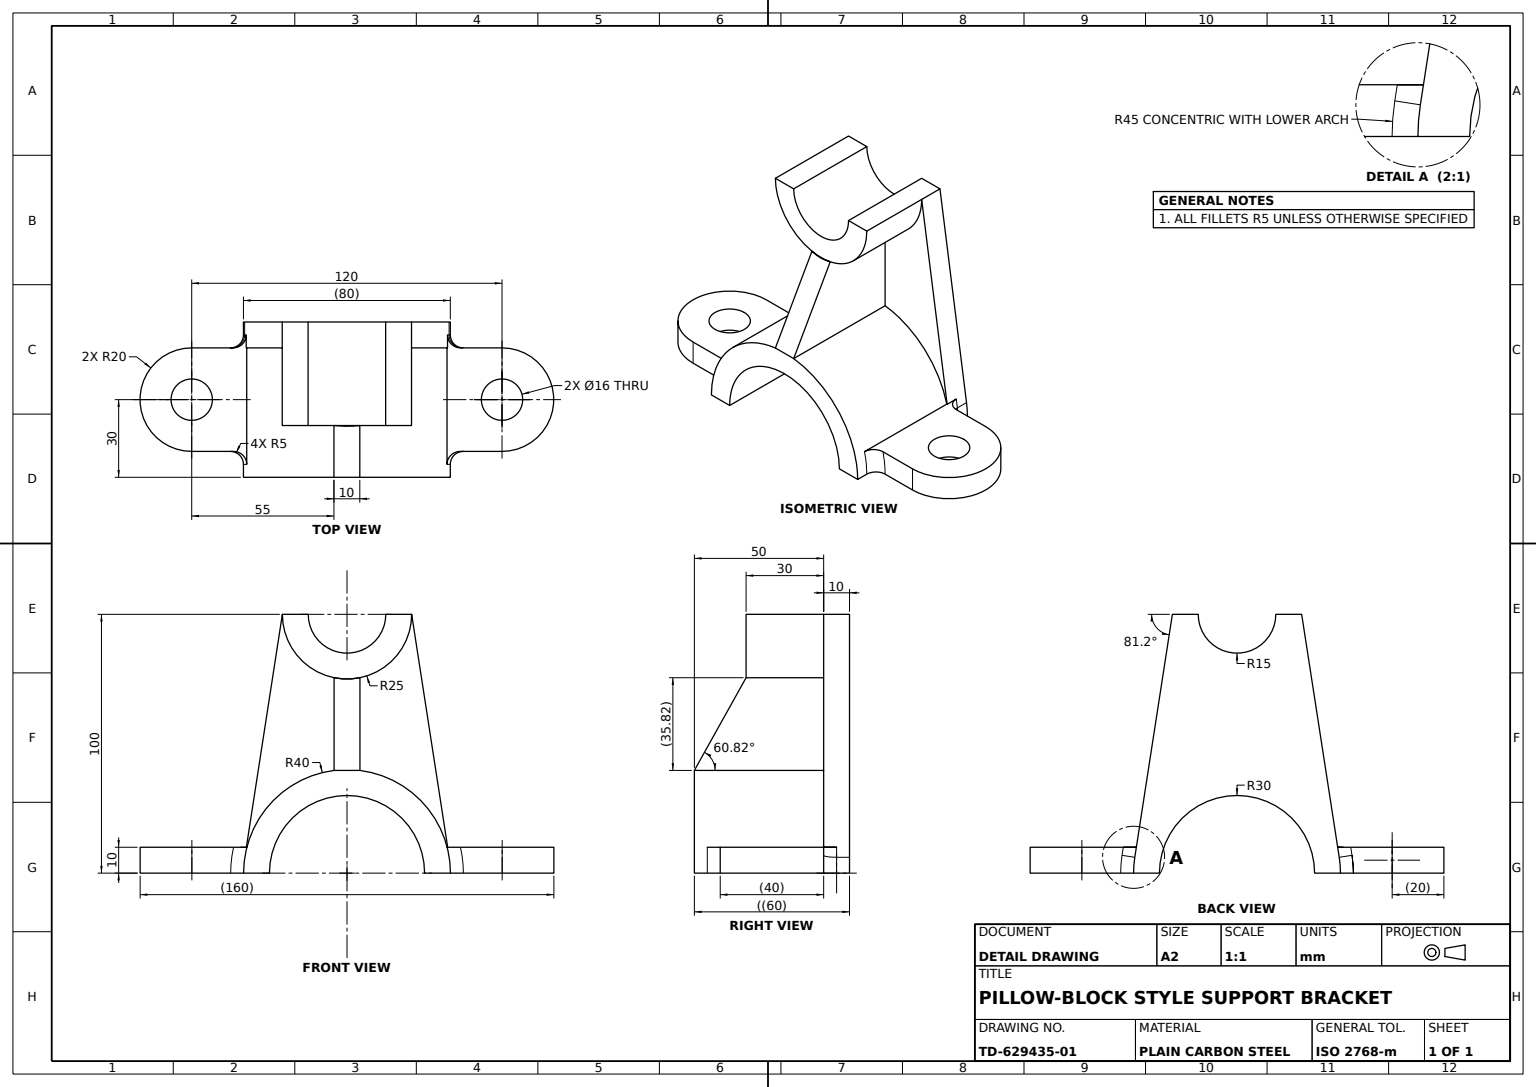
from build123d import *

# Parameters (mm, degrees)
BASE_BLOCK_DEPTH        = 50
UPRIGHT_BODY_DEPTH      = 30
SADDLE_FLANGE_DEPTH     = 10
SIDE_BOSS_1_DEPTH       = 10
SIDE_BOSS_2_DEPTH       = 10
MOUNTING_LUG_1_SKETCH_R = 8
MOUNTING_LUG_1_DEPTH    = 10
LUG_1_BOSS_SKETCH_W     = 40
LUG_1_BOSS_SKETCH_H     = 10
LUG_1_BOSS_DEPTH        = 5
LUG_1_FILLET_R5_R       = 5
MOUNTING_LUG_2_SKETCH_R = 8
MOUNTING_LUG_2_DEPTH    = 10
LUG_2_BOSS_SKETCH_W     = 40
LUG_2_BOSS_SKETCH_H     = 10
LUG_2_BOSS_DEPTH        = 5
LUG_2_FILLET_R5_R       = 5
SIDE_RIB_DEPTH          = 50
RIB_RELIEF_CUT_DEPTH    = 15


with BuildPart() as part:
    # Base Profile Sketch → Base Block (new body)
    with BuildSketch(Plane.XY):
        with BuildLine():
            Line((-40, 0), (-30, 0))
            ThreePointArc((-30, 0), (0, 30), (30, 0))
            Line((30, 0), (40, 0))
            ThreePointArc((40, 0), (0, 40), (-40, 0))
        make_face()
    extrude(amount=BASE_BLOCK_DEPTH)



with BuildPart() as body_2:
    # Upright Profile Sketch → Upright Body (new body)
    with BuildSketch(Plane.XY.offset(50)):
        with BuildLine():
            Line((-25, 100), (-15, 100))
            ThreePointArc((-15, 100), (0, 85), (15, 100))
            Line((15, 100), (25, 100))
            ThreePointArc((25, 100), (0, 75), (-25, 100))
        make_face()
    extrude(amount=-UPRIGHT_BODY_DEPTH)



with BuildPart() as body_3:
    # Saddle Flange Sketch → Saddle Flange (new body)
    with BuildSketch(Plane.XY.offset(50)):
        with BuildLine():
            Line((-25, 100), (-39.529411765, 6.117647059))
            ThreePointArc((-39.529411765, 6.117647059), (0, 40), (39.529411765, 6.117647059))
            Line((39.529411765, 6.117647059), (25, 100))
            ThreePointArc((25, 100), (0, 75), (-25, 100))
        make_face()
    extrude(amount=SADDLE_FLANGE_DEPTH)


with BuildPart() as body_2_1:
    add(body_2.part)

    add(body_3.part)  # Side Boss 1 merges body 3
    # Side Boss 1 Sketch → Side Boss 1 (add)
    with BuildSketch(Plane.XY.offset(50)):
        with BuildLine():
            Line((-15, 100), (-25, 100))
            ThreePointArc((-25, 100), (0, 75), (25, 100))
            Line((25, 100), (15, 100))
            ThreePointArc((15, 100), (0, 85), (-15, 100))
        make_face()
    extrude(amount=SIDE_BOSS_1_DEPTH)


with BuildPart() as part_1:
    add(part.part)

    add(body_2_1.part)  # Side Boss 2 merges body 2
    # Side Boss 2 Sketch → Side Boss 2 (add)
    with BuildSketch(Plane.XY.offset(50)):
        with BuildLine():
            Line((30, 0), (40, 0))
            ThreePointArc((40, 0), (0, 40), (-40, 0))
            Line((-40, 0), (-30, 0))
            ThreePointArc((-30, 0), (0, 30), (30, 0))
        make_face()
    extrude(amount=SIDE_BOSS_2_DEPTH)



with BuildPart() as body_2_2:
    # Mounting Lug 1 Sketch → Mounting Lug 1 (new body)
    with BuildSketch(Plane.XZ):
        with BuildLine():
            Line((-60, 50), (-40, 50))
            Line((-40, 50), (-40, 10))
            Line((-40, 10), (-60, 10))
            ThreePointArc((-60, 10), (-80, 30), (-60, 50))
        make_face()
        with Locations(Location((-60, 30, 0), (0, 0, 270))):
            Circle(MOUNTING_LUG_1_SKETCH_R, mode=Mode.SUBTRACT)
    extrude(amount=-MOUNTING_LUG_1_DEPTH)


with BuildPart() as part_2:
    add(part_1.part)

    add(body_2_2.part)  # Lug 1 Boss merges body 2 2
    # Lug 1 Boss Sketch → Lug 1 Boss (add)
    with BuildSketch(Plane(origin=(-40, 0, 0), x_dir=(0, 0, -1), z_dir=(1, 0, 0))):
        with Locations((-30, 5)):
            Rectangle(LUG_1_BOSS_SKETCH_W, LUG_1_BOSS_SKETCH_H)
    extrude(amount=LUG_1_BOSS_DEPTH)

    # Lug 1 Fillet R5
    lug_1_fillet_r5_edges = [part_2.edges().sort_by_distance(p)[0] for p in [
        (-39.228991597, 8.058823529, 50),
        (-39.681187851, 5.040171699, 10),
        (-39.88217942, 3.067859955, 50),
    ]]
    fillet(lug_1_fillet_r5_edges, radius=LUG_1_FILLET_R5_R)



with BuildPart() as body_2_3:
    # Mounting Lug 2 Sketch → Mounting Lug 2 (new body)
    with BuildSketch(Plane.XZ):
        with BuildLine():
            Line((60, 50), (40, 50))
            Line((40, 50), (40, 10))
            Line((40, 10), (60, 10))
            ThreePointArc((60, 10), (80, 30), (60, 50))
        make_face()
        with Locations(Location((60, 30, 0), (0, 0, 270))):
            Circle(MOUNTING_LUG_2_SKETCH_R, mode=Mode.SUBTRACT)
    extrude(amount=-MOUNTING_LUG_2_DEPTH)


with BuildPart() as part_3:
    add(part_2.part)

    add(body_2_3.part)  # Lug 2 Boss merges body 2 3
    # Lug 2 Boss Sketch → Lug 2 Boss (add)
    with BuildSketch(Plane.ZY.offset(-40)):
        with Locations((30, 5)):
            Rectangle(LUG_2_BOSS_SKETCH_W, LUG_2_BOSS_SKETCH_H)
    extrude(amount=LUG_2_BOSS_DEPTH)

    # Lug 2 Fillet R5
    lug_2_fillet_r5_edges = [part_3.edges().sort_by_distance(p)[0] for p in [
        (39.681187851, 5.040171699, 10),
        (39.88217942, 3.067859955, 50),
        (39.228991597, 8.058823529, 50),
    ]]
    fillet(lug_2_fillet_r5_edges, radius=LUG_2_FILLET_R5_R)

    # Side Rib Sketch → Side Rib (add)
    with BuildSketch(Plane(origin=(0, 0, 50), x_dir=(-1, 0, 0), z_dir=(0, 0, -1))):
        with BuildLine():
            Line((-5, 75.505102572), (-5, 39.686269666))
            ThreePointArc((-5, 39.686269666), (0, 40), (5, 39.686269666))
            Line((5, 39.686269666), (5, 75.505102572))
            ThreePointArc((5, 75.505102572), (0, 75), (-5, 75.505102572))
        make_face()
    extrude(amount=SIDE_RIB_DEPTH)

    # Rib Relief Cut Sketch → Rib Relief Cut (cut)
    with BuildSketch(Plane.ZY.offset(5)):
        Polygon((20, 75.505102572), (0, 39.686269666), (0, 75.505102572), align=None)
    extrude(amount=-RIB_RELIEF_CUT_DEPTH, mode=Mode.SUBTRACT)


solid = part_3.part
